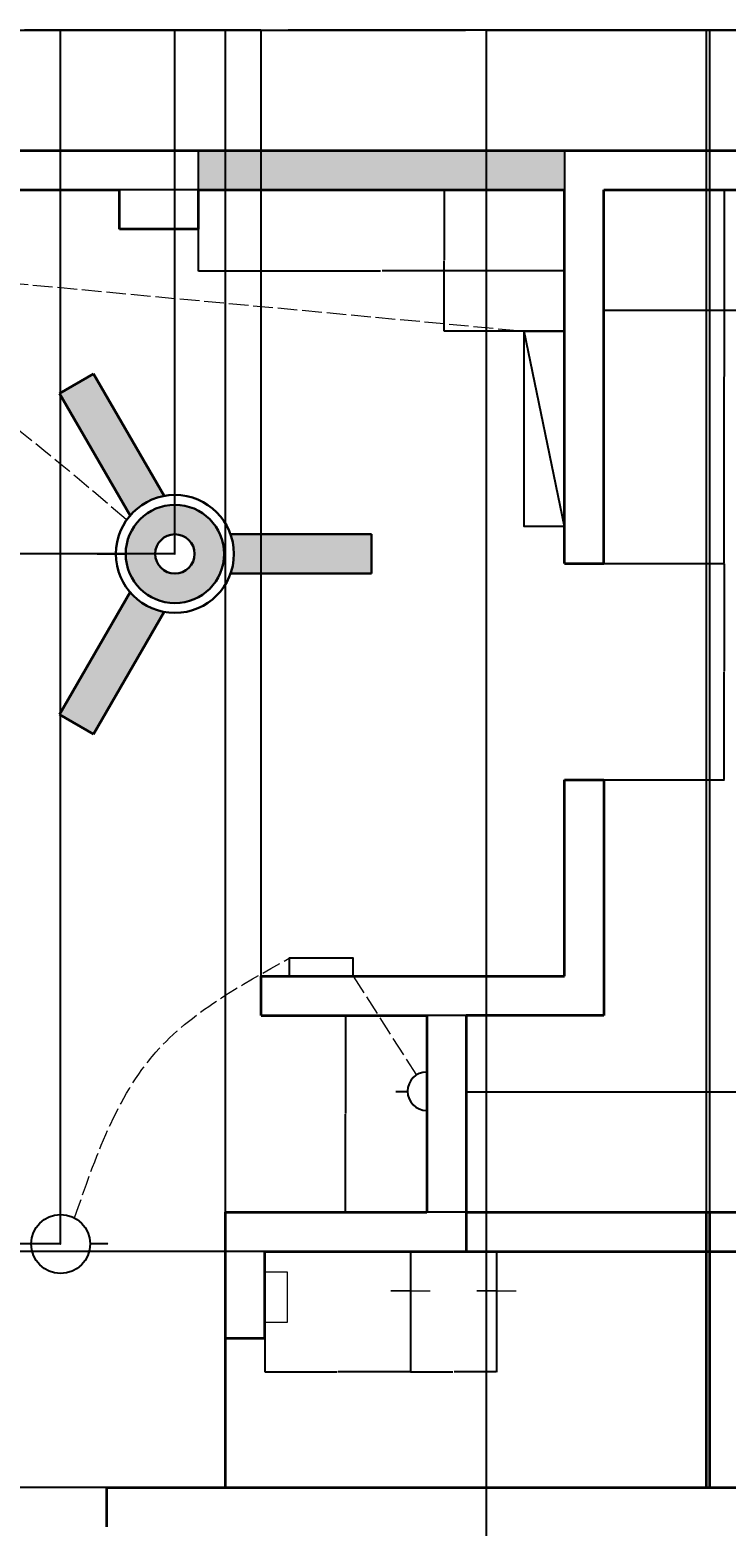
# Model space of a CAD drawing. Units: inches. Extents: x 2034 to 3646, y 962 to 2549.
# Tile 3 of 4: x 2683 to 3108, y 1636 to 2549. Entities that reach past the tile are written whole.
import ezdxf

# ---------------------------------------------------------------- set-up
doc = ezdxf.new("R2010")
doc.units = ezdxf.units.IN
doc.linetypes.add('ACAD_ISO02W100', pattern=[15, 12, -3])
for name, color, linetype, lineweight in [('A-ANNO-DIMS', 2, 'Continuous', 18), ('A-FLOR-FIXT', 9, 'Continuous', 18), ('A-GLAZ', 250, 'Continuous', 18), ('E-EQPM-FANS', 7, 'Continuous', 30), ('E-LITE-CTRL', 7, 'Continuous', 25), ('E-LITE-FIXT', 7, 'Continuous', 25), ('E-POWR-DEVC', 7, 'Continuous', 25)]:
    doc.layers.add(name, color=color, linetype=linetype, lineweight=lineweight)
for name, color, linetype, lineweight, true_color in [('A-GLAZ-PATT', 18, 'Continuous', 13, 0x000000), ('A-WALL', 203, 'Continuous', 35, 0xa780c2), ('E-LITE-WIRE', 103, 'ACAD_ISO02W100', 18, 0x6dc08b)]:
    doc.layers.add(name, color=color, linetype=linetype, lineweight=lineweight, true_color=true_color)
doc.styles.get("Standard").update_dxf_attribs({"font": 'arial.ttf'})
doc.dimstyles.get("Standard").update_dxf_attribs({"dimtxt": 0.18, "dimasz": 0.18, "dimexe": 0.18, "dimexo": 0.0625, "dimgap": 0.09, "dimtad": 0, "dimtih": 1, "dimtoh": 1, "dimdec": 4, "dimzin": 0, "dimdsep": 46, "dimtxsty": 'Standard', "dimcen": 0.09, "dimadec": 0, "dimazin": 0, "dimtfac": 1, "dimtdec": 4, "dimtofl": 0, "dimtmove": 0, "dimatfit": 3, "dimfxl": 1, "dimtolj": 1, "dimtzin": 0, "dimarcsym": 0})

# ---------------------------------------------------------------- blocks, each defined once
blk = doc.blocks.new('CEILING-FAN-3-BLADE')
h = blk.add_hatch(color=256)
h.dxf.hatch_style = 1
h.paths.add_polyline_path([(-49.61, 109.92), (-70.39, 97.92), (-27.36, 23.39, -0.171573), (-6.58, 35.39)])
h = blk.add_hatch(color=256)
h.dxf.hatch_style = 1
h.paths.add_polyline_path([(-30, 0, 1), (30, 0, 1)])
h.paths.add_polyline_path([(12, 0, -1), (-12, 0, -1)], flags=16)
h = blk.add_hatch(color=256)
h.dxf.hatch_style = 1
h.paths.add_polyline_path([(120, 12), (33.94, 12, -0.085164), (36, 0, -0.085164), (33.94, -12), (120, -12)])
h = blk.add_hatch(color=256)
h.dxf.hatch_style = 1
h.paths.add_polyline_path([(-6.58, -35.39, -0.171573), (-27.36, -23.39), (-70.39, -97.92), (-49.61, -109.92)])
for p, q in [((-70.39, 97.92), (-49.61, 109.92)), ((-49.61, 109.92), (-6.58, 35.39)), ((-27.36, 23.39), (-70.39, 97.92)), ((33.94, 12), (120, 12)), ((120, 12), (120, -12)), ((120, -12), (33.94, -12)), ((-70.39, -97.92), (-27.36, -23.39)), ((-6.58, -35.39), (-49.61, -109.92)), ((-49.61, -109.92), (-70.39, -97.92))]:
    blk.add_line(p, q)
for radius in [36, 30, 12]:
    blk.add_circle((0, 0), radius)
blk = doc.blocks.new('WALL-FITTING-T')
for p, q in [((0, 0), (0, -24)), ((0, -24), (-12, -24)), ((-12, -24), (12, -24))]:
    blk.add_line(p, q)
blk = doc.blocks.new('*D4')
at = {"layer": 'A-ANNO-DIMS', "color": 0, "lineweight": -2, "transparency": 16777216}
for p, q in [((2108.2, 2475.7), (2108.2, 2549.27)), ((2108.38, 2549.09), (2839.85, 2549.09)), ((3572.02, 2549.09), (2840.55, 2549.09)), ((3572.2, 2475.7), (3572.2, 2549.27))]:
    blk.add_line(p, q, dxfattribs=at)
at = {"layer": 'A-ANNO-DIMS', "color": 0, "transparency": 16777216}
for points in [[(2108.38, 2549.12), (2108.38, 2549.06), (2108.2, 2549.09)], [(3572.02, 2549.12), (3572.02, 2549.06), (3572.2, 2549.09)]]:
    blk.add_solid(points, dxfattribs=at)
at = {"layer": 'Defpoints', "color": 0, "transparency": 16777216}
for p in [(3572.2, 2549.09), (2108.2, 2475.64), (3572.2, 2475.64)]:
    blk.add_point(p, dxfattribs=at)
at = {"layer": 'A-ANNO-DIMS', "color": 0, "transparency": 16777216, "insert": (2840.2, 2549.09), "char_height": 0.18, "attachment_point": 5}
blk.add_mtext('\\A1;1464', dxfattribs=at)
blk = doc.blocks.new('*D11')
at = {"layer": 'A-ANNO-DIMS', "color": 0, "lineweight": -2, "transparency": 16777216}
for p, q in [((3033.12, 2451.58), (3033.12, 2378.01)), ((3548.2, 2451.58), (3548.2, 2378.01)), ((3033.3, 2378.19), (3290.28, 2378.19)), ((3548.02, 2378.19), (3291.04, 2378.19))]:
    blk.add_line(p, q, dxfattribs=at)
at = {"layer": 'A-ANNO-DIMS', "color": 0, "transparency": 16777216}
for points in [[(3033.3, 2378.22), (3033.3, 2378.16), (3033.12, 2378.19)], [(3548.02, 2378.22), (3548.02, 2378.16), (3548.2, 2378.19)]]:
    blk.add_solid(points, dxfattribs=at)
at = {"layer": 'Defpoints', "color": 0, "transparency": 16777216}
for p in [(3033.12, 2451.64), (3548.2, 2451.64), (3033.12, 2378.19)]:
    blk.add_point(p, dxfattribs=at)
at = {"layer": 'A-ANNO-DIMS', "color": 0, "transparency": 16777216, "insert": (3290.66, 2378.19), "char_height": 0.18, "attachment_point": 5}
blk.add_mtext('\\A1;515.1', dxfattribs=at)
blk = doc.blocks.new('*D12')
at = {"layer": 'A-ANNO-DIMS', "color": 0, "lineweight": -2, "transparency": 16777216}
for p, q in [((3033.19, 2451.64), (3106.75, 2451.64)), ((3106.57, 2451.46), (3106.57, 2337.82)), ((3106.57, 2223.82), (3106.57, 2337.46)), ((3033.19, 2223.64), (3106.75, 2223.64))]:
    blk.add_line(p, q, dxfattribs=at)
at = {"layer": 'A-ANNO-DIMS', "color": 0, "transparency": 16777216}
for points in [[(3106.54, 2451.46), (3106.6, 2451.46), (3106.57, 2451.64)], [(3106.54, 2223.82), (3106.6, 2223.82), (3106.57, 2223.64)]]:
    blk.add_solid(points, dxfattribs=at)
at = {"layer": 'Defpoints', "color": 0, "transparency": 16777216}
for p in [(3033.12, 2451.64), (3033.12, 2223.64), (3106.57, 2223.64)]:
    blk.add_point(p, dxfattribs=at)
at = {"layer": 'A-ANNO-DIMS', "color": 0, "transparency": 16777216, "insert": (3106.57, 2337.64), "char_height": 0.18, "attachment_point": 5}
blk.add_mtext('\\A1;228', dxfattribs=at)
blk = doc.blocks.new('*D13')
at = {"layer": 'A-ANNO-DIMS', "color": 0, "lineweight": -2, "transparency": 16777216}
for p, q in [((3033.19, 2223.64), (3106.75, 2223.64)), ((3106.57, 2223.46), (3106.57, 2157.82)), ((3106.57, 2091.82), (3106.57, 2157.46)), ((3033.19, 2091.64), (3106.75, 2091.64))]:
    blk.add_line(p, q, dxfattribs=at)
at = {"layer": 'A-ANNO-DIMS', "color": 0, "transparency": 16777216}
for points in [[(3106.54, 2223.46), (3106.6, 2223.46), (3106.57, 2223.64)], [(3106.54, 2091.82), (3106.6, 2091.82), (3106.57, 2091.64)]]:
    blk.add_solid(points, dxfattribs=at)
at = {"layer": 'Defpoints', "color": 0, "transparency": 16777216}
for p in [(3033.12, 2223.64), (3033.12, 2091.64), (3106.57, 2091.64)]:
    blk.add_point(p, dxfattribs=at)
at = {"layer": 'A-ANNO-DIMS', "color": 0, "transparency": 16777216, "insert": (3106.57, 2157.64), "char_height": 0.18, "attachment_point": 5}
blk.add_mtext('\\A1;132', dxfattribs=at)
blk = doc.blocks.new('*D15')
at = {"layer": 'A-ANNO-DIMS', "color": 0, "lineweight": -2, "transparency": 16777216}
for p, q in [((2588.2, 1971.7), (2588.2, 2549.27)), ((2588.38, 2549.09), (2705.7, 2549.09)), ((2823.95, 2549.09), (2706.63, 2549.09)), ((2824.13, 1971.7), (2824.13, 2549.27))]:
    blk.add_line(p, q, dxfattribs=at)
at = {"layer": 'A-ANNO-DIMS', "color": 0, "transparency": 16777216}
for points in [[(2588.38, 2549.12), (2588.38, 2549.06), (2588.2, 2549.09)], [(2823.95, 2549.12), (2823.95, 2549.06), (2824.13, 2549.09)]]:
    blk.add_solid(points, dxfattribs=at)
at = {"layer": 'Defpoints', "color": 0, "transparency": 16777216}
for p in [(2824.13, 2549.09), (2588.2, 1971.64), (2824.13, 1971.64)]:
    blk.add_point(p, dxfattribs=at)
at = {"layer": 'A-ANNO-DIMS', "color": 0, "transparency": 16777216, "insert": (2706.16, 2549.09), "char_height": 0.18, "attachment_point": 5}
blk.add_mtext('\\A1;235.93', dxfattribs=at)
blk = doc.blocks.new('*D16')
at = {"layer": 'A-ANNO-DIMS', "color": 0, "lineweight": -2, "transparency": 16777216}
for p, q in [((2588.2, 1635.7), (2588.2, 2549.27)), ((2588.38, 2549.09), (2935.91, 2549.09)), ((3284.02, 2549.09), (2936.49, 2549.09)), ((3284.2, 1635.7), (3284.2, 2549.27))]:
    blk.add_line(p, q, dxfattribs=at)
at = {"layer": 'A-ANNO-DIMS', "color": 0, "transparency": 16777216}
for points in [[(2588.38, 2549.12), (2588.38, 2549.06), (2588.2, 2549.09)], [(3284.02, 2549.12), (3284.02, 2549.06), (3284.2, 2549.09)]]:
    blk.add_solid(points, dxfattribs=at)
at = {"layer": 'Defpoints', "color": 0, "transparency": 16777216}
for p in [(3284.2, 2549.09), (2588.2, 1635.64), (3284.2, 1635.64)]:
    blk.add_point(p, dxfattribs=at)
at = {"layer": 'A-ANNO-DIMS', "color": 0, "transparency": 16777216, "insert": (2936.2, 2549.09), "char_height": 0.18, "attachment_point": 5}
blk.add_mtext('\\A1;696', dxfattribs=at)
blk = doc.blocks.new('*D20')
at = {"layer": 'A-ANNO-DIMS', "color": 0, "lineweight": -2, "transparency": 16777216}
for p, q in [((3300.28, 1803.64), (2034.57, 1803.64)), ((2034.75, 1803.46), (2034.75, 1731.82)), ((2034.75, 1659.82), (2034.75, 1731.46)), ((3300.28, 1659.64), (2034.57, 1659.64))]:
    blk.add_line(p, q, dxfattribs=at)
at = {"layer": 'A-ANNO-DIMS', "color": 0, "transparency": 16777216}
for points in [[(2034.72, 1803.46), (2034.78, 1803.46), (2034.75, 1803.64)], [(2034.72, 1659.82), (2034.78, 1659.82), (2034.75, 1659.64)]]:
    blk.add_solid(points, dxfattribs=at)
at = {"layer": 'Defpoints', "color": 0, "transparency": 16777216}
for p in [(2034.75, 1803.64), (3300.34, 1803.64), (3300.34, 1659.64)]:
    blk.add_point(p, dxfattribs=at)
at = {"layer": 'A-ANNO-DIMS', "color": 0, "transparency": 16777216, "insert": (2034.75, 1731.64), "char_height": 0.18, "attachment_point": 5}
blk.add_mtext('\\A1;144', dxfattribs=at)
blk = doc.blocks.new('*D21')
at = {"layer": 'A-ANNO-DIMS', "color": 0, "lineweight": -2, "transparency": 16777216}
for p, q in [((2802.42, 1659.7), (2802.42, 2549.27)), ((2802.6, 2549.09), (2948.73, 2549.09)), ((3095.65, 2549.09), (2949.52, 2549.09)), ((3095.83, 1659.7), (3095.83, 2549.27))]:
    blk.add_line(p, q, dxfattribs=at)
at = {"layer": 'A-ANNO-DIMS', "color": 0, "transparency": 16777216}
for points in [[(2802.6, 2549.12), (2802.6, 2549.06), (2802.42, 2549.09)], [(3095.65, 2549.12), (3095.65, 2549.06), (3095.83, 2549.09)]]:
    blk.add_solid(points, dxfattribs=at)
at = {"layer": 'Defpoints', "color": 0, "transparency": 16777216}
for p in [(3095.83, 2549.09), (2802.42, 1659.64), (3095.83, 1659.64)]:
    blk.add_point(p, dxfattribs=at)
at = {"layer": 'A-ANNO-DIMS', "color": 0, "transparency": 16777216, "insert": (2949.12, 2549.09), "char_height": 0.18, "attachment_point": 5}
blk.add_mtext('\\A1;293.4', dxfattribs=at)
blk = doc.blocks.new('*D22')
at = {"layer": 'A-ANNO-DIMS', "color": 0, "lineweight": -2, "transparency": 16777216}
for p, q in [((3097.83, 1659.7), (3097.83, 2549.27)), ((3098.01, 2549.09), (3198.69, 2549.09)), ((3300.16, 2549.09), (3199.48, 2549.09)), ((3300.34, 1659.7), (3300.34, 2549.27))]:
    blk.add_line(p, q, dxfattribs=at)
at = {"layer": 'A-ANNO-DIMS', "color": 0, "transparency": 16777216}
for points in [[(3098.01, 2549.12), (3098.01, 2549.06), (3097.83, 2549.09)], [(3300.16, 2549.12), (3300.16, 2549.06), (3300.34, 2549.09)]]:
    blk.add_solid(points, dxfattribs=at)
at = {"layer": 'Defpoints', "color": 0, "transparency": 16777216}
for p in [(3300.34, 2549.09), (3097.83, 1659.64), (3300.34, 1659.64)]:
    blk.add_point(p, dxfattribs=at)
at = {"layer": 'A-ANNO-DIMS', "color": 0, "transparency": 16777216, "insert": (3199.08, 2549.09), "char_height": 0.18, "attachment_point": 5}
blk.add_mtext('\\A1;202.5', dxfattribs=at)
blk = doc.blocks.new('*D23')
at = {"layer": 'A-ANNO-DIMS', "color": 0, "lineweight": -2, "transparency": 16777216}
for p, q in [((2915.14, 1803.58), (2915.14, 1730.01)), ((2967.75, 1803.58), (2967.75, 1730.01)), ((2915.32, 1730.19), (2941.05, 1730.19)), ((2967.57, 1730.19), (2941.84, 1730.19))]:
    blk.add_line(p, q, dxfattribs=at)
at = {"layer": 'A-ANNO-DIMS', "color": 0, "transparency": 16777216}
for points in [[(2915.32, 1730.22), (2915.32, 1730.16), (2915.14, 1730.19)], [(2967.57, 1730.22), (2967.57, 1730.16), (2967.75, 1730.19)]]:
    blk.add_solid(points, dxfattribs=at)
at = {"layer": 'Defpoints', "color": 0, "transparency": 16777216}
for p in [(2915.14, 1803.64), (2967.75, 1803.64), (2915.14, 1730.19)]:
    blk.add_point(p, dxfattribs=at)
at = {"layer": 'A-ANNO-DIMS', "color": 0, "transparency": 16777216, "insert": (2941.44, 1730.19), "char_height": 0.18, "attachment_point": 5}
blk.add_mtext('\\A1;52.62', dxfattribs=at)
blk = doc.blocks.new('*D26')
at = {"layer": 'A-ANNO-DIMS', "color": 0, "lineweight": -2, "transparency": 16777216}
for p, q in [((2587.47, 2222.22), (2587.47, 2549.27)), ((2587.65, 2549.09), (2679.2, 2549.09)), ((2771.3, 2549.09), (2679.76, 2549.09)), ((2771.48, 2229.49), (2771.48, 2549.27))]:
    blk.add_line(p, q, dxfattribs=at)
at = {"layer": 'A-ANNO-DIMS', "color": 0, "transparency": 16777216}
for points in [[(2587.65, 2549.12), (2587.65, 2549.06), (2587.47, 2549.09)], [(2771.3, 2549.12), (2771.3, 2549.06), (2771.48, 2549.09)]]:
    blk.add_solid(points, dxfattribs=at)
at = {"layer": 'Defpoints', "color": 0, "transparency": 16777216}
for p in [(2771.48, 2549.09), (2771.48, 2229.42), (2587.47, 2222.15)]:
    blk.add_point(p, dxfattribs=at)
at = {"layer": 'A-ANNO-DIMS', "color": 0, "transparency": 16777216, "insert": (2679.48, 2549.09), "char_height": 0.18, "attachment_point": 5}
blk.add_mtext('\\A1;184', dxfattribs=at)
blk = doc.blocks.new('*D28')
at = {"layer": 'A-ANNO-DIMS', "color": 0, "lineweight": -2, "transparency": 16777216}
for p, q in [((2785.69, 2451.64), (2034.57, 2451.64)), ((2034.75, 2451.46), (2034.75, 2340.71)), ((2034.75, 2229.6), (2034.75, 2340.35)), ((2771.42, 2229.42), (2034.57, 2229.42))]:
    blk.add_line(p, q, dxfattribs=at)
at = {"layer": 'A-ANNO-DIMS', "color": 0, "transparency": 16777216}
for points in [[(2034.72, 2451.46), (2034.78, 2451.46), (2034.75, 2451.64)], [(2034.72, 2229.6), (2034.78, 2229.6), (2034.75, 2229.42)]]:
    blk.add_solid(points, dxfattribs=at)
at = {"layer": 'Defpoints', "color": 0, "transparency": 16777216}
for p in [(2034.75, 2451.64), (2785.75, 2451.64), (2771.48, 2229.42)]:
    blk.add_point(p, dxfattribs=at)
at = {"layer": 'A-ANNO-DIMS', "color": 0, "transparency": 16777216, "insert": (2034.75, 2340.53), "char_height": 0.18, "attachment_point": 5}
blk.add_mtext('\\A1;222.2', dxfattribs=at)
blk = doc.blocks.new('*D33')
at = {"layer": 'A-ANNO-DIMS', "color": 0, "lineweight": -2, "transparency": 16777216}
for p, q in [((2961.58, 1396.49), (2961.58, 2549.27)), ((2961.76, 2549.09), (3122.5, 2549.09)), ((3284.02, 2549.09), (3123.28, 2549.09)), ((3284.2, 1304.99), (3284.2, 2549.27))]:
    blk.add_line(p, q, dxfattribs=at)
at = {"layer": 'A-ANNO-DIMS', "color": 0, "transparency": 16777216}
for points in [[(2961.76, 2549.12), (2961.76, 2549.06), (2961.58, 2549.09)], [(3284.02, 2549.12), (3284.02, 2549.06), (3284.2, 2549.09)]]:
    blk.add_solid(points, dxfattribs=at)
at = {"layer": 'Defpoints', "color": 0, "transparency": 16777216}
for p in [(3284.2, 2549.09), (2961.58, 1396.43), (3284.2, 1304.92)]:
    blk.add_point(p, dxfattribs=at)
at = {"layer": 'A-ANNO-DIMS', "color": 0, "transparency": 16777216, "insert": (3122.89, 2549.09), "char_height": 0.18, "attachment_point": 5}
blk.add_mtext('\\A1;322.6', dxfattribs=at)
blk = doc.blocks.new('*D39')
at = {"layer": 'A-ANNO-DIMS', "color": 0, "lineweight": -2, "transparency": 16777216}
for p, q in [((2785.75, 2475.58), (2785.75, 2402.01)), ((3009.12, 2475.58), (3009.12, 2402.01)), ((2785.93, 2402.19), (2896.97, 2402.19)), ((3008.94, 2402.19), (2897.9, 2402.19))]:
    blk.add_line(p, q, dxfattribs=at)
at = {"layer": 'A-ANNO-DIMS', "color": 0, "transparency": 16777216}
for points in [[(2785.93, 2402.22), (2785.93, 2402.16), (2785.75, 2402.19)], [(3008.94, 2402.22), (3008.94, 2402.16), (3009.12, 2402.19)]]:
    blk.add_solid(points, dxfattribs=at)
at = {"layer": 'Defpoints', "color": 0, "transparency": 16777216}
for p in [(2785.75, 2475.64), (3009.12, 2475.64), (2785.75, 2402.19)]:
    blk.add_point(p, dxfattribs=at)
at = {"layer": 'A-ANNO-DIMS', "color": 0, "transparency": 16777216, "insert": (2897.44, 2402.19), "char_height": 0.18, "attachment_point": 5}
blk.add_mtext('\\A1;223.38', dxfattribs=at)
blk = doc.blocks.new('*D45')
at = {"layer": 'A-ANNO-DIMS', "color": 0, "lineweight": -2, "transparency": 16777216}
for p, q in [((2701.68, 1808.27), (2034.57, 1808.27)), ((2034.75, 1808.09), (2034.75, 1734.14)), ((2034.75, 1659.82), (2034.75, 1733.77)), ((2802.36, 1659.64), (2034.57, 1659.64))]:
    blk.add_line(p, q, dxfattribs=at)
at = {"layer": 'A-ANNO-DIMS', "color": 0, "transparency": 16777216}
for points in [[(2034.72, 1808.09), (2034.78, 1808.09), (2034.75, 1808.27)], [(2034.72, 1659.82), (2034.78, 1659.82), (2034.75, 1659.64)]]:
    blk.add_solid(points, dxfattribs=at)
at = {"layer": 'Defpoints', "color": 0, "transparency": 16777216}
for p in [(2034.75, 1808.27), (2701.74, 1808.27), (2802.42, 1659.64)]:
    blk.add_point(p, dxfattribs=at)
at = {"layer": 'A-ANNO-DIMS', "color": 0, "transparency": 16777216, "insert": (2034.75, 1733.96), "char_height": 0.18, "attachment_point": 5}
blk.add_mtext('\\A1;148.63', dxfattribs=at)
blk = doc.blocks.new('*D46')
at = {"layer": 'A-ANNO-DIMS', "color": 0, "lineweight": -2, "transparency": 16777216}
for p, q in [((2701.74, 1808.33), (2701.74, 2549.27)), ((2701.92, 2549.09), (2751.62, 2549.09)), ((2802.24, 2549.09), (2752.54, 2549.09)), ((2802.42, 1827.7), (2802.42, 2549.27))]:
    blk.add_line(p, q, dxfattribs=at)
at = {"layer": 'A-ANNO-DIMS', "color": 0, "transparency": 16777216}
for points in [[(2701.92, 2549.12), (2701.92, 2549.06), (2701.74, 2549.09)], [(2802.24, 2549.12), (2802.24, 2549.06), (2802.42, 2549.09)]]:
    blk.add_solid(points, dxfattribs=at)
at = {"layer": 'Defpoints', "color": 0, "transparency": 16777216}
for p in [(2701.74, 2549.09), (2802.42, 1827.64), (2701.74, 1808.27)]:
    blk.add_point(p, dxfattribs=at)
at = {"layer": 'A-ANNO-DIMS', "color": 0, "transparency": 16777216, "insert": (2752.08, 2549.09), "char_height": 0.18, "attachment_point": 5}
blk.add_mtext('\\A1;100.68', dxfattribs=at)
blk = doc.blocks.new('*D47')
at = {"layer": 'A-ANNO-DIMS', "color": 0, "lineweight": -2, "transparency": 16777216}
for p, q in [((2826.42, 1803.58), (2826.42, 1730.01)), ((2915.14, 1803.58), (2915.14, 1730.01)), ((2826.6, 1730.19), (2870.4, 1730.19)), ((2914.96, 1730.19), (2871.16, 1730.19))]:
    blk.add_line(p, q, dxfattribs=at)
at = {"layer": 'A-ANNO-DIMS', "color": 0, "transparency": 16777216}
for points in [[(2826.6, 1730.22), (2826.6, 1730.16), (2826.42, 1730.19)], [(2914.96, 1730.22), (2914.96, 1730.16), (2915.14, 1730.19)]]:
    blk.add_solid(points, dxfattribs=at)
at = {"layer": 'Defpoints', "color": 0, "transparency": 16777216}
for p in [(2826.42, 1803.64), (2915.14, 1803.64), (2826.42, 1730.19)]:
    blk.add_point(p, dxfattribs=at)
at = {"layer": 'A-ANNO-DIMS', "color": 0, "transparency": 16777216, "insert": (2870.78, 1730.19), "char_height": 0.18, "attachment_point": 5}
blk.add_mtext('\\A1;88.71', dxfattribs=at)
blk = doc.blocks.new('*D50')
at = {"layer": 'A-ANNO-DIMS', "color": 0, "lineweight": -2, "transparency": 16777216}
for p, q in [((2949.06, 1947.64), (2875.49, 1947.64)), ((2875.67, 1947.46), (2875.67, 1887.82)), ((2875.67, 1827.82), (2875.67, 1887.46)), ((2949.06, 1827.64), (2875.49, 1827.64))]:
    blk.add_line(p, q, dxfattribs=at)
at = {"layer": 'A-ANNO-DIMS', "color": 0, "transparency": 16777216}
for points in [[(2875.64, 1947.46), (2875.7, 1947.46), (2875.67, 1947.64)], [(2875.64, 1827.82), (2875.7, 1827.82), (2875.67, 1827.64)]]:
    blk.add_solid(points, dxfattribs=at)
at = {"layer": 'Defpoints', "color": 0, "transparency": 16777216}
for p in [(2875.67, 1947.64), (2949.12, 1947.64), (2949.12, 1827.64)]:
    blk.add_point(p, dxfattribs=at)
at = {"layer": 'A-ANNO-DIMS', "color": 0, "transparency": 16777216, "insert": (2875.67, 1887.64), "char_height": 0.18, "attachment_point": 5}
blk.add_mtext('\\A1;120', dxfattribs=at)
blk = doc.blocks.new('*D51')
at = {"layer": 'A-ANNO-DIMS', "color": 0, "lineweight": -2, "transparency": 16777216}
for p, q in [((2949.12, 1827.7), (2949.12, 1901.27)), ((2949.3, 1901.09), (3124.34, 1901.09)), ((3300.16, 1901.09), (3125.12, 1901.09)), ((3300.34, 1827.7), (3300.34, 1901.27))]:
    blk.add_line(p, q, dxfattribs=at)
at = {"layer": 'A-ANNO-DIMS', "color": 0, "transparency": 16777216}
for points in [[(2949.3, 1901.12), (2949.3, 1901.06), (2949.12, 1901.09)], [(3300.16, 1901.12), (3300.16, 1901.06), (3300.34, 1901.09)]]:
    blk.add_solid(points, dxfattribs=at)
at = {"layer": 'Defpoints', "color": 0, "transparency": 16777216}
for p in [(3300.34, 1901.09), (2949.12, 1827.64), (3300.34, 1827.64)]:
    blk.add_point(p, dxfattribs=at)
at = {"layer": 'A-ANNO-DIMS', "color": 0, "transparency": 16777216, "insert": (3124.73, 1901.09), "char_height": 0.18, "attachment_point": 5}
blk.add_mtext('\\A1;351.2', dxfattribs=at)
blk = doc.blocks.new('*D56')
at = {"layer": 'A-ANNO-DIMS', "color": 0, "lineweight": -2, "transparency": 16777216}
for p, q in [((3009.06, 2451.64), (2935.49, 2451.64)), ((2935.67, 2451.46), (2935.67, 2408.71)), ((2935.67, 2365.6), (2935.67, 2408.35)), ((3009.06, 2365.42), (2935.49, 2365.42))]:
    blk.add_line(p, q, dxfattribs=at)
at = {"layer": 'A-ANNO-DIMS', "color": 0, "transparency": 16777216}
for points in [[(2935.64, 2451.46), (2935.7, 2451.46), (2935.67, 2451.64)], [(2935.64, 2365.6), (2935.7, 2365.6), (2935.67, 2365.42)]]:
    blk.add_solid(points, dxfattribs=at)
at = {"layer": 'Defpoints', "color": 0, "transparency": 16777216}
for p in [(2935.67, 2451.64), (3009.12, 2451.64), (3009.12, 2365.42)]:
    blk.add_point(p, dxfattribs=at)
at = {"layer": 'A-ANNO-DIMS', "color": 0, "transparency": 16777216, "insert": (2935.67, 2408.53), "char_height": 0.18, "attachment_point": 5}
blk.add_mtext('\\A1;86.22', dxfattribs=at)
blk = doc.blocks.new('*D65')
at = {"layer": 'A-ANNO-DIMS', "color": 0, "lineweight": -2, "transparency": 16777216}
for p, q in [((2723.99, 2229.42), (2741.3, 2229.42)), ((2771.39, 2229.42), (2771.57, 2229.42)), ((2771.48, 2229.33), (2771.48, 2229.51))]:
    blk.add_line(p, q, dxfattribs=at)
at = {"layer": 'A-ANNO-DIMS', "color": 0, "transparency": 16777216}
blk.add_solid([(2741.3, 2229.45), (2741.3, 2229.39), (2741.48, 2229.42)], dxfattribs=at)
at = {"layer": 'Defpoints', "color": 0, "transparency": 16777216}
for p in [(2741.48, 2229.42), (2801.48, 2229.42)]:
    blk.add_point(p, dxfattribs=at)
at = {"layer": 'A-ANNO-DIMS', "color": 0, "transparency": 16777216, "insert": (2723.48, 2229.42), "char_height": 0.18, "attachment_point": 5}
blk.add_mtext('\\A1;4X ∅60', dxfattribs=at)
blk = doc.blocks.new('*D73')
at = {"layer": 'A-ANNO-DIMS', "color": 0, "lineweight": -2, "transparency": 16777216}
for p, q in [((2701.65, 1808.27), (2701.83, 1808.27)), ((2701.74, 1808.18), (2701.74, 1808.36)), ((2730.54, 1808.27), (2719.92, 1808.27))]:
    blk.add_line(p, q, dxfattribs=at)
at = {"layer": 'A-ANNO-DIMS', "color": 0, "transparency": 16777216}
blk.add_solid([(2719.92, 1808.3), (2719.92, 1808.24), (2719.74, 1808.27)], dxfattribs=at)
at = {"layer": 'Defpoints', "color": 0, "transparency": 16777216}
for p in [(2683.74, 1808.27), (2719.74, 1808.27)]:
    blk.add_point(p, dxfattribs=at)
at = {"layer": 'A-ANNO-DIMS', "color": 0, "transparency": 16777216, "insert": (2730.85, 1808.27), "char_height": 0.18, "attachment_point": 5}
blk.add_mtext('\\A1;∅36', dxfattribs=at)
blk = doc.blocks.new('*D77')
at = {"layer": 'A-ANNO-DIMS', "color": 0, "lineweight": -2, "transparency": 16777216}
for p, q in [((2906.36, 1901.35), (2913.22, 1901.4)), ((2925.04, 1901.48), (2925.22, 1901.48)), ((2925.13, 1901.39), (2925.13, 1901.57))]:
    blk.add_line(p, q, dxfattribs=at)
at = {"layer": 'A-ANNO-DIMS', "color": 0, "transparency": 16777216}
blk.add_solid([(2913.22, 1901.43), (2913.22, 1901.37), (2913.4, 1901.4)], dxfattribs=at)
at = {"layer": 'Defpoints', "color": 0, "transparency": 16777216}
for p in [(2913.4, 1901.4), (2925.13, 1901.48)]:
    blk.add_point(p, dxfattribs=at)
at = {"layer": 'A-ANNO-DIMS', "color": 0, "transparency": 16777216, "insert": (2905.88, 1901.35), "char_height": 0.18, "attachment_point": 5}
blk.add_mtext('\\A1;R11.73', dxfattribs=at)

msp = doc.modelspace()

# ---------------------------------------------------------------- hatches: boundary and pattern name
at = {"layer": 'A-GLAZ-PATT'}
h = msp.add_hatch(color=256, dxfattribs=at)
h.dxf.hatch_style = 1
h.paths.add_polyline_path([(3009.1244, 2475.6388), (2785.7486, 2475.6388), (2785.7486, 2451.6388), (3009.1244, 2451.6388)])

# ---------------------------------------------------------------- linework, layer by layer
at = {"layer": 'A-FLOR-FIXT'}
msp.add_lwpolyline([(2826.4216, 1760.5938), (2840.1927, 1760.5938), (2840.1927, 1790.9746), (2826.4216, 1790.9746)], close=True, dxfattribs=at)
at = {"layer": 'A-GLAZ'}
for p, q in [((2785.7486, 2451.6388), (2785.7486, 2475.6388)), ((2785.7486, 2475.6388), (3009.1244, 2475.6388)), ((3009.1244, 2451.6388), (3009.1244, 2475.6388)), ((2785.7486, 2451.6388), (3009.1244, 2451.6388))]:
    msp.add_line(p, q, dxfattribs=at)
at = {"layer": 'A-WALL'}
for p, q in [((2295.4968, 2451.6388), (2737.7486, 2451.6388)), ((2737.7486, 2427.6388), (2737.7486, 2451.6388)), ((2785.7486, 2451.6388), (2785.7486, 2427.6388)), ((2785.7486, 2451.6388), (3009.1244, 2451.6388)), ((3009.1244, 2223.6388), (3009.1244, 2451.6388)), ((3033.1244, 2223.6388), (3033.1244, 2451.6388)), ((3033.1244, 2451.6388), (3284.1976, 2451.6388)), ((2785.7486, 2427.6388), (2737.7486, 2427.6388)), ((3009.1244, 2223.6388), (3033.1244, 2223.6388)), ((3009.1244, 1971.6388), (3009.1244, 2091.6388)), ((3009.1244, 2091.6388), (3033.1244, 2091.6388)), ((3033.1244, 2091.6388), (3033.1244, 1947.6388)), ((2824.1305, 1947.6388), (2824.1305, 1971.6388)), ((2824.1305, 1971.6388), (3009.1244, 1971.6388)), ((2824.1305, 1947.6388), (2925.1305, 1947.6388)), ((2925.1305, 1947.6388), (2925.1305, 1827.6388)), ((3033.1244, 1947.6388), (2949.1244, 1947.6388)), ((2949.1244, 1947.6388), (2949.1244, 1803.6388)), ((2802.4216, 1827.6388), (2925.1305, 1827.6388)), ((2802.4216, 1659.6388), (2802.4216, 1827.6388)), ((2949.1244, 1827.6388), (3300.3398, 1827.6388)), ((3095.8265, 1659.6388), (3095.8265, 1827.6388)), ((3097.8265, 1659.6388), (3097.8265, 1827.6388)), ((2826.4216, 1803.6388), (3300.3398, 1803.6388)), ((2826.4216, 1750.8218), (2826.4216, 1803.6388)), ((2802.4216, 1750.8218), (2826.4216, 1750.8218)), ((2729.8258, 1659.6388), (3300.3398, 1659.6388)), ((2729.8258, 1659.6388), (2729.8258, 1635.6388))]:
    msp.add_line(p, q, dxfattribs=at)
msp.add_lwpolyline([(2108.1976, 1407.6388), (2108.1976, 2475.6388), (3308.1976, 2475.6388)], dxfattribs=at)
at = {"layer": 'E-LITE-CTRL'}
msp.add_lwpolyline([(2841.2975, 1971.6388), (2880.2785, 1971.6388), (2880.2785, 1982.6083), (2841.2975, 1982.6083)], close=True, dxfattribs=at)
at = {"layer": 'E-LITE-FIXT'}
msp.add_line((3009.1244, 2246.2683), (2984.5836, 2365.4191), dxfattribs=at)
msp.add_lwpolyline([(3009.1244, 2246.2683), (2984.5836, 2246.2683), (2984.5836, 2365.4191), (3009.1244, 2365.4191)], close=True, dxfattribs=at)
msp.add_circle((2701.738, 1808.2715), 18, dxfattribs=at)
at = {"layer": 'E-LITE-WIRE'}
for p, q in [((2386.1907, 2421.6388), (2984.5836, 2365.4191)), ((2880.2785, 1971.6388), (2918.812, 1911.3647))]:
    msp.add_line(p, q, dxfattribs=at)
for points, knots in [([(2386.1907, 2421.6388), (2450.6467, 2409.6898), (2584.5763, 2384.8618), (2688.3336, 2296.2606), (2742.1558, 2250.3004)], [0, 0, 0, 0, 193.13075599, 401.29592099, 401.29592099, 401.29592099, 401.29592099]), ([(2710.2662, 1824.1229), (2723.0372, 1861.0798), (2747.0853, 1930.6704), (2811.2216, 1966.0278), (2841.2975, 1982.6083)], [0, 0, 0, 0, 112.72403461, 212.26176192, 212.26176192, 212.26176192, 212.26176192])]:
    msp.add_open_spline(points, degree=3, knots=knots, dxfattribs=at)
at = {"layer": 'E-POWR-DEVC'}
msp.add_arc((2925.1305, 1901.4813), 11.7306, 90, 270, dxfattribs=at)

# ---------------------------------------------------------------- block references
at = {"layer": 'A-FLOR-FIXT'}
for p in [(2915.1363, 1803.6388), (2967.7523, 1803.6388)]:
    msp.add_blockref('WALL-FITTING-T', p, dxfattribs=at)
at = {"layer": 'E-EQPM-FANS'}
msp.add_blockref('CEILING-FAN-3-BLADE', (2771.4839, 2229.423), dxfattribs=at)

# ---------------------------------------------------------------- dimensions: what is measured, and where the dimension line sits
at = {"layer": 'A-ANNO-DIMS'}
for base, p1, p2, override, picture, middle in [((3572.1976, 2549.0888), (2108.1976, 2475.6388), (3572.1976, 2475.6388), {"dimdec": 0, "dimlfac": 1, "dimrnd": 0, "dimzin": 0, "dimdsep": 46, "dimlunit": 2}, '*D4', (2840.1976, 2549.0888)), ((2771.4839, 2549.0888), (2587.4667, 2222.1542), (2771.4839, 2229.423), {"dimdec": 0, "dimlfac": 1, "dimrnd": 0, "dimzin": 0, "dimdsep": 46, "dimlunit": 2}, '*D26', (2679.4753, 2549.0888)), ((2824.1305, 2549.0888), (2588.1976, 1971.6388), (2824.1305, 1971.6388), {"dimdec": 2, "dimlfac": 1, "dimrnd": 0, "dimzin": 0, "dimdsep": 46, "dimlunit": 2}, '*D15', (2706.1641, 2549.0888)), ((3284.1976, 2549.0888), (2588.1976, 1635.6388), (3284.1976, 1635.6388), {"dimdec": 0, "dimlfac": 1, "dimrnd": 0, "dimzin": 0, "dimdsep": 46, "dimlunit": 2}, '*D16', (2936.1976, 2549.0888)), ((2701.738, 2549.0888), (2802.4216, 1827.6388), (2701.738, 1808.2715), {"dimdec": 2, "dimlfac": 1, "dimrnd": 0, "dimzin": 0, "dimdsep": 46, "dimlunit": 2}, '*D46', (2752.0798, 2549.0888)), ((3095.8265, 2549.0888), (2802.4216, 1659.6388), (3095.8265, 1659.6388), {"dimdec": 1, "dimlfac": 1, "dimrnd": 0, "dimzin": 0, "dimdsep": 46, "dimlunit": 2}, '*D21', (2949.124, 2549.0888)), ((3284.1976, 2549.0888), (2961.5838, 1396.4302), (3284.1976, 1304.9248), {"dimdec": 1, "dimlfac": 1, "dimrnd": 0, "dimzin": 0, "dimdsep": 46, "dimlunit": 2}, '*D33', (3122.8907, 2549.0888)), ((3300.3398, 2549.0888), (3097.8265, 1659.6388), (3300.3398, 1659.6388), {"dimdec": 1, "dimlfac": 1, "dimrnd": 0, "dimzin": 0, "dimdsep": 46, "dimlunit": 2}, '*D22', (3199.0831, 2549.0888)), ((3300.3398, 1901.0888), (2949.1244, 1827.6388), (3300.3398, 1827.6388), {"dimdec": 1, "dimlfac": 1, "dimrnd": 0, "dimzin": 0, "dimdsep": 46, "dimlunit": 2}, '*D51', (3124.7321, 1901.0888))]:
    dim = msp.add_linear_dim(base=base, p1=p1, p2=p2, dimstyle='Standard', override=override, dxfattribs=at)
    dim.commit()
    dim.dimension.update_dxf_attribs({"geometry": picture, "text_midpoint": middle})
for base, p1, p2, angle, override, picture, middle in [((2785.7486, 2402.1888), (3009.1244, 2475.6388), (2785.7486, 2475.6388), 180, {"dimdec": 2, "dimlfac": 1, "dimrnd": 0, "dimzin": 0, "dimdsep": 46, "dimlunit": 2}, '*D39', (2897.4365, 2402.1888)), ((2034.7476, 2451.6388), (2771.4839, 2229.423), (2785.7486, 2451.6388), 90, {"dimdec": 1, "dimlfac": 1, "dimrnd": 0, "dimzin": 0, "dimdsep": 46, "dimlunit": 2}, '*D28', (2034.7476, 2340.5309)), ((2935.6744, 2451.6388), (3009.1244, 2365.4191), (3009.1244, 2451.6388), 90, {"dimdec": 2, "dimlfac": 1, "dimrnd": 0, "dimzin": 0, "dimdsep": 46, "dimlunit": 2}, '*D56', (2935.6744, 2408.5289)), ((3033.1244, 2378.1888), (3548.1976, 2451.6388), (3033.1244, 2451.6388), 180, {"dimdec": 1, "dimlfac": 1, "dimrnd": 0, "dimzin": 0, "dimdsep": 46, "dimlunit": 2}, '*D11', (3290.661, 2378.1888)), ((3106.5744, 2223.6388), (3033.1244, 2451.6388), (3033.1244, 2223.6388), 270, {"dimdec": 0, "dimlfac": 1, "dimrnd": 0, "dimzin": 0, "dimdsep": 46, "dimlunit": 2}, '*D12', (3106.5744, 2337.6388)), ((3106.5744, 2091.6388), (3033.1244, 2223.6388), (3033.1244, 2091.6388), 270, {"dimdec": 0, "dimlfac": 1, "dimrnd": 0, "dimzin": 0, "dimdsep": 46, "dimlunit": 2}, '*D13', (3106.5744, 2157.6388)), ((2875.6744, 1947.6388), (2949.1244, 1827.6388), (2949.1244, 1947.6388), 90, {"dimdec": 0, "dimlfac": 1, "dimrnd": 0, "dimzin": 0, "dimdsep": 46, "dimlunit": 2}, '*D50', (2875.6744, 1887.6388)), ((2034.7476, 1808.2715), (2802.4216, 1659.6388), (2701.738, 1808.2715), 90, {"dimdec": 2, "dimlfac": 1, "dimrnd": 0, "dimzin": 0, "dimdsep": 46, "dimlunit": 2}, '*D45', (2034.7476, 1733.9551)), ((2034.7476, 1803.6388), (3300.3398, 1659.6388), (3300.3398, 1803.6388), 90, {"dimdec": 0, "dimlfac": 1, "dimrnd": 0, "dimzin": 0, "dimdsep": 46, "dimlunit": 2}, '*D20', (2034.7476, 1731.6388)), ((2826.4216, 1730.1888), (2915.1363, 1803.6388), (2826.4216, 1803.6388), 180, {"dimdec": 2, "dimlfac": 1, "dimrnd": 0, "dimzin": 0, "dimdsep": 46, "dimlunit": 2}, '*D47', (2870.7789, 1730.1888)), ((2915.1363, 1730.1888), (2967.7523, 1803.6388), (2915.1363, 1803.6388), 180, {"dimdec": 2, "dimlfac": 1, "dimrnd": 0, "dimzin": 0, "dimdsep": 46, "dimlunit": 2}, '*D23', (2941.4443, 1730.1888))]:
    dim = msp.add_linear_dim(base=base, p1=p1, p2=p2, angle=angle, dimstyle='Standard', override=override, dxfattribs=at)
    dim.commit()
    dim.dimension.update_dxf_attribs({"geometry": picture, "text_midpoint": middle})
dim = msp.add_diameter_dim_2p(p1=(2801.4839, 2229.423), p2=(2741.4839, 2229.423), text='4X <>', dimstyle='Standard', override={"dimdec": 0, "dimlfac": 1, "dimrnd": 0, "dimzin": 0, "dimdsep": 46, "dimlunit": 2}, dxfattribs=at)
dim.commit()
dim.dimension.update_dxf_attribs({"geometry": '*D65', "text_midpoint": (2723.4839, 2229.423), "dimtype": 163})
dim = msp.add_radius_dim(center=(2925.1305, 1901.4813), mpoint=(2913.4002, 1901.3986), dimstyle='Standard', override={"dimdec": 2, "dimlfac": 1, "dimrnd": 0, "dimzin": 0, "dimdsep": 46, "dimlunit": 2}, dxfattribs=at)
dim.commit()
dim.dimension.update_dxf_attribs({"geometry": '*D77', "text_midpoint": (2906.3621, 1901.349), "dimtype": 164})
dim = msp.add_diameter_dim_2p(p1=(2683.738, 1808.272), p2=(2719.738, 1808.271), dimstyle='Standard', override={"dimdec": 0, "dimlfac": 1, "dimrnd": 0, "dimzin": 0, "dimdsep": 46, "dimlunit": 2}, dxfattribs=at)
dim.commit()
dim.dimension.update_dxf_attribs({"geometry": '*D73', "text_midpoint": (2730.538, 1808.2707), "dimtype": 163})

doc.saveas('drawing.dxf')
